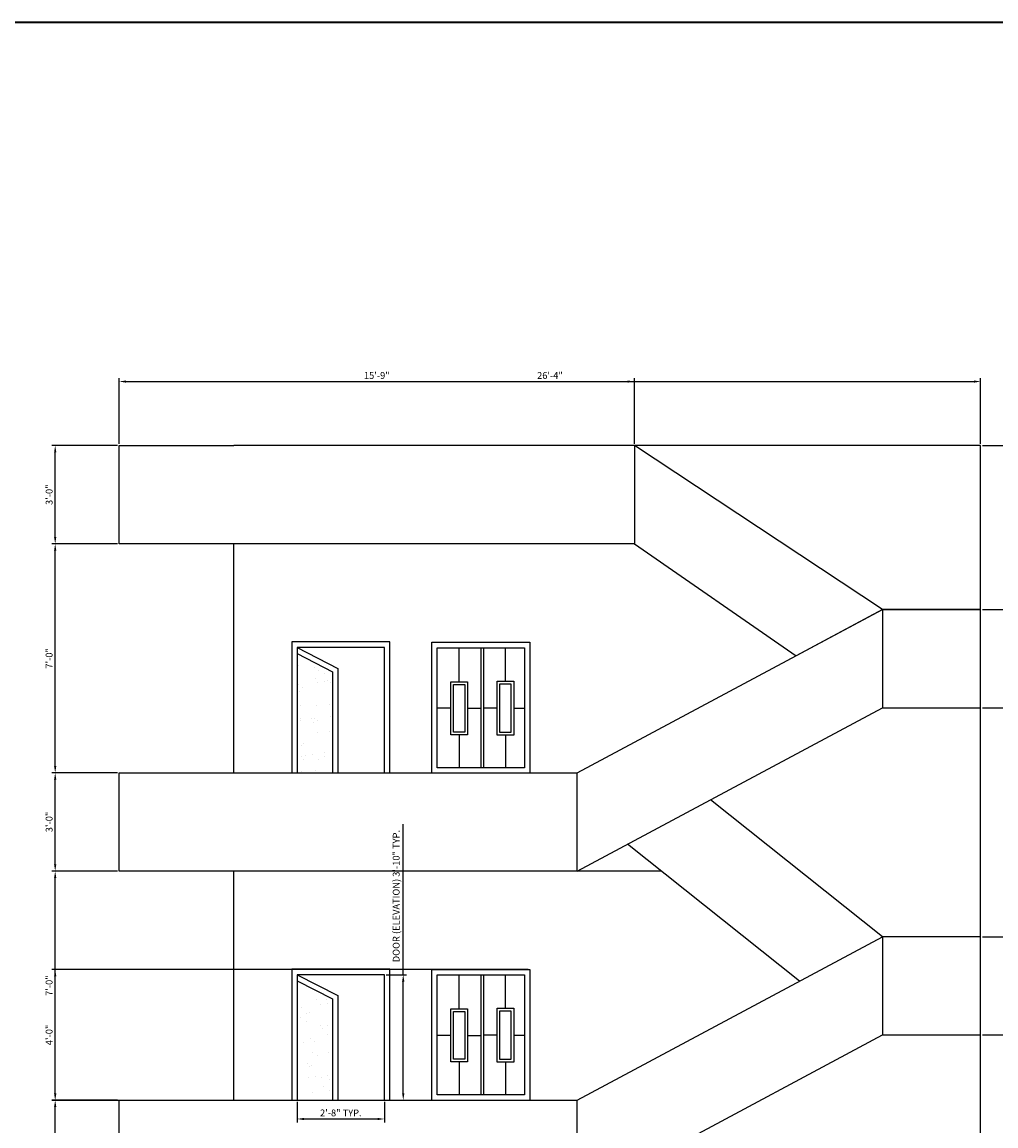
# Model space of a CAD drawing. Units: inches. Extents: x 2020 to 7901, y 1581 to 3943.
# Tile 7 of 17: x 2315 to 2672, y 2663 to 3067. Entities that reach past the tile are written whole.
import ezdxf

# ---------------------------------------------------------------- set-up
doc = ezdxf.new("R2010")
doc.units = ezdxf.units.IN
for name, color, linetype, lineweight in [('A-ANNO-DIMS', 2, 'Continuous', 18), ('A-ANNO-TTLB', 7, 'Continuous', 35), ('A-ELEV', 7, 'Continuous', 25), ('A-ELEV-PATT', 8, 'Continuous', 13)]:
    doc.layers.add(name, color=color, linetype=linetype, lineweight=lineweight)
doc.styles.get("Standard").update_dxf_attribs({"font": 'arial.ttf'})
doc.dimstyles.new('ISO-25', dxfattribs={"dimtxt": 2.5, "dimasz": 2.5, "dimexe": 1.25, "dimexo": 0.625, "dimtad": 1, "dimdec": 1, "dimlunit": 3, "dimtxsty": 'Standard', "dimcen": 2.5, "dimadec": 0, "dimazin": 0, "dimtfac": 1, "dimtdec": 1, "dimtmove": 0, "dimatfit": 3, "dimfxl": 1, "dimarcsym": 0})
pattern_1 = [(37.5, (-52.601, -26.04), (-0.320006, 9.788265), [0, -7.7216, 0, -8.636, 0, -8.255]), (7.5, (-52.601, -26.04), (8.990466, 14.3365), [0, -4.1656, 0, -6.9596, 0, -2.667]), (327.5, (-58.849, -26.04), (15.819847, 0.028744), [0, -2.54, 0, -9.144, 0, -11.938]), (317.5, (-58.85, -26.04), (15.27113, 4.458586), [0, -1.27, 0, -5.9944, 0, -6.858])]

# ---------------------------------------------------------------- blocks, each defined once
blk = doc.blocks.new('ELEV-DOOR')
for p, q in [((32, 46), (0, 46)), ((0, 46), (0, 0)), ((0, 46), (14.91, 38.33)), ((32, 0), (32, 46)), ((14.91, 38.33), (14.91, 0))]:
    blk.add_line(p, q)
blk = doc.blocks.new('*D29')
at = {"layer": 'A-ANNO-DIMS', "color": 0, "lineweight": -2, "transparency": 16777216}
for p, q in [((2454.54, 2717.95), (2454.54, 2773.1)), ((2448.26, 2717.95), (2455.79, 2717.95)), ((2454.54, 2674.45), (2454.54, 2715.45)), ((2448.26, 2671.95), (2455.79, 2671.95))]:
    blk.add_line(p, q, dxfattribs=at)
at = {"layer": 'A-ANNO-DIMS', "color": 0, "transparency": 16777216}
for points in [[(2454.12, 2715.45), (2454.96, 2715.45), (2454.54, 2717.95)], [(2454.12, 2674.45), (2454.96, 2674.45), (2454.54, 2671.95)]]:
    blk.add_solid(points, dxfattribs=at)
at = {"layer": 'DEFPOINTS', "color": 0, "transparency": 16777216}
for p in [(2447.64, 2717.95), (2454.54, 2717.95), (2447.64, 2671.95)]:
    blk.add_point(p, dxfattribs=at)
at = {"layer": 'A-ANNO-DIMS', "color": 0, "transparency": 16777216, "insert": (2452.27, 2746.77), "char_height": 2.5, "attachment_point": 5, "rotation": 90}
blk.add_mtext('DOOR (ELEVATION) 3\'-10" TYP.', dxfattribs=at)
blk = doc.blocks.new('*D30')
at = {"layer": 'A-ANNO-DIMS', "color": 0, "lineweight": -2, "transparency": 16777216}
for p, q in [((2415.64, 2671.32), (2415.64, 2663.8)), ((2447.64, 2671.32), (2447.64, 2663.8)), ((2418.14, 2665.05), (2445.14, 2665.05))]:
    blk.add_line(p, q, dxfattribs=at)
at = {"layer": 'A-ANNO-DIMS', "color": 0, "transparency": 16777216}
for points in [[(2418.14, 2665.46), (2418.14, 2664.63), (2415.64, 2665.05)], [(2445.14, 2665.46), (2445.14, 2664.63), (2447.64, 2665.05)]]:
    blk.add_solid(points, dxfattribs=at)
at = {"layer": 'DEFPOINTS', "color": 0, "transparency": 16777216}
for p in [(2415.64, 2671.95), (2447.64, 2671.95), (2447.64, 2665.05)]:
    blk.add_point(p, dxfattribs=at)
at = {"layer": 'A-ANNO-DIMS', "color": 0, "transparency": 16777216, "insert": (2431.64, 2666.95), "char_height": 2.5, "attachment_point": 5}
blk.add_mtext('2\'-8" TYP.', dxfattribs=at)
blk = doc.blocks.new('*D62')
at = {"layer": 'A-ANNO-DIMS', "color": 0, "lineweight": -2, "transparency": 16777216}
for p, q in [((2350.36, 2912.57), (2350.36, 2936.7)), ((2352.86, 2935.45), (2663.86, 2935.45)), ((2666.36, 2912.57), (2666.36, 2936.7))]:
    blk.add_line(p, q, dxfattribs=at)
at = {"layer": 'A-ANNO-DIMS', "color": 0, "transparency": 16777216}
for points in [[(2352.86, 2935.86), (2352.86, 2935.03), (2350.36, 2935.45)], [(2663.86, 2935.86), (2663.86, 2935.03), (2666.36, 2935.45)]]:
    blk.add_solid(points, dxfattribs=at)
at = {"layer": 'DEFPOINTS', "color": 0, "transparency": 16777216}
for p in [(2666.36, 2935.45), (2350.36, 2911.95), (2666.36, 2911.95)]:
    blk.add_point(p, dxfattribs=at)
at = {"layer": 'A-ANNO-DIMS', "color": 0, "transparency": 16777216, "insert": (2508.36, 2937.35), "char_height": 2.5, "attachment_point": 5}
blk.add_mtext('26\'-4"', dxfattribs=at)
blk = doc.blocks.new('*D63')
at = {"layer": 'A-ANNO-DIMS', "color": 0, "lineweight": -2, "transparency": 16777216}
for p, q in [((2666.99, 2911.95), (2728.83, 2911.95)), ((2727.58, 2490.45), (2727.58, 2909.45)), ((2666.99, 2487.95), (2728.83, 2487.95))]:
    blk.add_line(p, q, dxfattribs=at)
at = {"layer": 'A-ANNO-DIMS', "color": 0, "transparency": 16777216}
for points in [[(2727.17, 2909.45), (2728, 2909.45), (2727.58, 2911.95)], [(2727.17, 2490.45), (2728, 2490.45), (2727.58, 2487.95)]]:
    blk.add_solid(points, dxfattribs=at)
at = {"layer": 'DEFPOINTS', "color": 0, "transparency": 16777216}
for p in [(2666.36, 2911.95), (2727.58, 2911.95), (2666.36, 2487.95)]:
    blk.add_point(p, dxfattribs=at)
at = {"layer": 'A-ANNO-DIMS', "color": 0, "transparency": 16777216, "insert": (2725.68, 2699.95), "char_height": 2.5, "attachment_point": 5, "rotation": 90}
blk.add_mtext('35\'-4"', dxfattribs=at)
blk = doc.blocks.new('*D68')
at = {"layer": 'A-ANNO-DIMS', "color": 0, "lineweight": -2, "transparency": 16777216}
for p, q in [((2349.74, 2671.95), (2325.61, 2671.95)), ((2326.86, 2638.45), (2326.86, 2669.45)), ((2349.74, 2635.95), (2325.61, 2635.95))]:
    blk.add_line(p, q, dxfattribs=at)
at = {"layer": 'A-ANNO-DIMS', "color": 0, "transparency": 16777216}
for points in [[(2326.45, 2669.45), (2327.28, 2669.45), (2326.86, 2671.95)], [(2326.45, 2638.45), (2327.28, 2638.45), (2326.86, 2635.95)]]:
    blk.add_solid(points, dxfattribs=at)
at = {"layer": 'DEFPOINTS', "color": 0, "transparency": 16777216}
for p in [(2326.86, 2671.95), (2350.36, 2671.95), (2350.36, 2635.95)]:
    blk.add_point(p, dxfattribs=at)
at = {"layer": 'A-ANNO-DIMS', "color": 0, "transparency": 16777216, "insert": (2324.96, 2653.95), "char_height": 2.5, "attachment_point": 5, "rotation": 90}
blk.add_mtext('3\'-0"', dxfattribs=at)
blk = doc.blocks.new('*D69')
at = {"layer": 'A-ANNO-DIMS', "color": 0, "lineweight": -2, "transparency": 16777216}
for p, q in [((2349.74, 2755.95), (2325.61, 2755.95)), ((2326.86, 2674.45), (2326.86, 2753.45)), ((2349.74, 2671.95), (2325.61, 2671.95))]:
    blk.add_line(p, q, dxfattribs=at)
at = {"layer": 'A-ANNO-DIMS', "color": 0, "transparency": 16777216}
for points in [[(2326.45, 2753.45), (2327.28, 2753.45), (2326.86, 2755.95)], [(2326.45, 2674.45), (2327.28, 2674.45), (2326.86, 2671.95)]]:
    blk.add_solid(points, dxfattribs=at)
at = {"layer": 'DEFPOINTS', "color": 0, "transparency": 16777216}
for p in [(2326.86, 2755.95), (2350.36, 2755.95), (2350.36, 2671.95)]:
    blk.add_point(p, dxfattribs=at)
at = {"layer": 'A-ANNO-DIMS', "color": 0, "transparency": 16777216, "insert": (2324.96, 2713.95), "char_height": 2.5, "attachment_point": 5, "rotation": 90}
blk.add_mtext('7\'-0"', dxfattribs=at)
blk = doc.blocks.new('*D70')
at = {"layer": 'A-ANNO-DIMS', "color": 0, "lineweight": -2, "transparency": 16777216}
for p, q in [((2349.74, 2791.95), (2325.61, 2791.95)), ((2326.86, 2758.45), (2326.86, 2789.45)), ((2349.74, 2755.95), (2325.61, 2755.95))]:
    blk.add_line(p, q, dxfattribs=at)
at = {"layer": 'A-ANNO-DIMS', "color": 0, "transparency": 16777216}
for points in [[(2326.45, 2789.45), (2327.28, 2789.45), (2326.86, 2791.95)], [(2326.45, 2758.45), (2327.28, 2758.45), (2326.86, 2755.95)]]:
    blk.add_solid(points, dxfattribs=at)
at = {"layer": 'DEFPOINTS', "color": 0, "transparency": 16777216}
for p in [(2326.86, 2791.95), (2350.36, 2791.95), (2350.36, 2755.95)]:
    blk.add_point(p, dxfattribs=at)
at = {"layer": 'A-ANNO-DIMS', "color": 0, "transparency": 16777216, "insert": (2324.96, 2773.95), "char_height": 2.5, "attachment_point": 5, "rotation": 90}
blk.add_mtext('3\'-0"', dxfattribs=at)
blk = doc.blocks.new('*D71')
at = {"layer": 'A-ANNO-DIMS', "color": 0, "lineweight": -2, "transparency": 16777216}
for p, q in [((2349.74, 2875.95), (2325.61, 2875.95)), ((2326.86, 2794.45), (2326.86, 2873.45)), ((2349.74, 2791.95), (2325.61, 2791.95))]:
    blk.add_line(p, q, dxfattribs=at)
at = {"layer": 'A-ANNO-DIMS', "color": 0, "transparency": 16777216}
for points in [[(2326.45, 2873.45), (2327.28, 2873.45), (2326.86, 2875.95)], [(2326.45, 2794.45), (2327.28, 2794.45), (2326.86, 2791.95)]]:
    blk.add_solid(points, dxfattribs=at)
at = {"layer": 'DEFPOINTS', "color": 0, "transparency": 16777216}
for p in [(2326.86, 2875.95), (2350.36, 2875.95), (2350.36, 2791.95)]:
    blk.add_point(p, dxfattribs=at)
at = {"layer": 'A-ANNO-DIMS', "color": 0, "transparency": 16777216, "insert": (2324.96, 2833.95), "char_height": 2.5, "attachment_point": 5, "rotation": 90}
blk.add_mtext('7\'-0"', dxfattribs=at)
blk = doc.blocks.new('*D72')
at = {"layer": 'A-ANNO-DIMS', "color": 0, "lineweight": -2, "transparency": 16777216}
for p, q in [((2349.74, 2911.95), (2325.61, 2911.95)), ((2326.86, 2878.45), (2326.86, 2909.45)), ((2349.74, 2875.95), (2325.61, 2875.95))]:
    blk.add_line(p, q, dxfattribs=at)
at = {"layer": 'A-ANNO-DIMS', "color": 0, "transparency": 16777216}
for points in [[(2326.45, 2909.45), (2327.28, 2909.45), (2326.86, 2911.95)], [(2326.45, 2878.45), (2327.28, 2878.45), (2326.86, 2875.95)]]:
    blk.add_solid(points, dxfattribs=at)
at = {"layer": 'DEFPOINTS', "color": 0, "transparency": 16777216}
for p in [(2326.86, 2911.95), (2350.36, 2911.95), (2350.36, 2875.95)]:
    blk.add_point(p, dxfattribs=at)
at = {"layer": 'A-ANNO-DIMS', "color": 0, "transparency": 16777216, "insert": (2324.96, 2893.95), "char_height": 2.5, "attachment_point": 5, "rotation": 90}
blk.add_mtext('3\'-0"', dxfattribs=at)
blk = doc.blocks.new('*D150')
at = {"layer": 'A-ANNO-DIMS', "color": 0, "lineweight": -2, "transparency": 16777216}
for p, q in [((2666.99, 2695.85), (2728.83, 2695.85)), ((2727.58, 2614.35), (2727.58, 2693.35)), ((2666.99, 2611.85), (2728.83, 2611.85))]:
    blk.add_line(p, q, dxfattribs=at)
at = {"layer": 'A-ANNO-DIMS', "color": 0, "transparency": 16777216}
for points in [[(2727.17, 2693.35), (2728, 2693.35), (2727.58, 2695.85)], [(2727.17, 2614.35), (2728, 2614.35), (2727.58, 2611.85)]]:
    blk.add_solid(points, dxfattribs=at)
at = {"layer": 'DEFPOINTS', "color": 0, "transparency": 16777216}
for p in [(2666.36, 2695.85), (2727.58, 2695.85), (2666.36, 2611.85)]:
    blk.add_point(p, dxfattribs=at)
at = {"layer": 'A-ANNO-DIMS', "color": 0, "transparency": 16777216, "insert": (2725.68, 2653.85), "char_height": 2.5, "attachment_point": 5, "rotation": 90}
blk.add_mtext('7\'-0"', dxfattribs=at)
blk = doc.blocks.new('*D151')
at = {"layer": 'A-ANNO-DIMS', "color": 0, "lineweight": -2, "transparency": 16777216}
for p, q in [((2666.99, 2731.85), (2728.83, 2731.85)), ((2727.58, 2698.35), (2727.58, 2729.35)), ((2666.99, 2695.85), (2728.83, 2695.85))]:
    blk.add_line(p, q, dxfattribs=at)
at = {"layer": 'A-ANNO-DIMS', "color": 0, "transparency": 16777216}
for points in [[(2727.17, 2729.35), (2728, 2729.35), (2727.58, 2731.85)], [(2727.17, 2698.35), (2728, 2698.35), (2727.58, 2695.85)]]:
    blk.add_solid(points, dxfattribs=at)
at = {"layer": 'DEFPOINTS', "color": 0, "transparency": 16777216}
for p in [(2666.36, 2731.85), (2727.58, 2731.85), (2666.36, 2695.85)]:
    blk.add_point(p, dxfattribs=at)
at = {"layer": 'A-ANNO-DIMS', "color": 0, "transparency": 16777216, "insert": (2725.68, 2713.85), "char_height": 2.5, "attachment_point": 5, "rotation": 90}
blk.add_mtext('3\'-0"', dxfattribs=at)
blk = doc.blocks.new('*D152')
at = {"layer": 'A-ANNO-DIMS', "color": 0, "lineweight": -2, "transparency": 16777216}
for p, q in [((2666.99, 2815.83), (2728.83, 2815.83)), ((2727.58, 2734.35), (2727.58, 2813.33)), ((2666.99, 2731.85), (2728.83, 2731.85))]:
    blk.add_line(p, q, dxfattribs=at)
at = {"layer": 'A-ANNO-DIMS', "color": 0, "transparency": 16777216}
for points in [[(2727.17, 2813.33), (2728, 2813.33), (2727.58, 2815.83)], [(2727.17, 2734.35), (2728, 2734.35), (2727.58, 2731.85)]]:
    blk.add_solid(points, dxfattribs=at)
at = {"layer": 'DEFPOINTS', "color": 0, "transparency": 16777216}
for p in [(2666.36, 2815.83), (2727.58, 2815.83), (2666.36, 2731.85)]:
    blk.add_point(p, dxfattribs=at)
at = {"layer": 'A-ANNO-DIMS', "color": 0, "transparency": 16777216, "insert": (2725.68, 2773.84), "char_height": 2.5, "attachment_point": 5, "rotation": 90}
blk.add_mtext('7\'-0"', dxfattribs=at)
blk = doc.blocks.new('*D153')
at = {"layer": 'A-ANNO-DIMS', "color": 0, "lineweight": -2, "transparency": 16777216}
for p, q in [((2666.99, 2851.83), (2728.83, 2851.83)), ((2727.58, 2818.33), (2727.58, 2849.33)), ((2666.99, 2815.83), (2728.83, 2815.83))]:
    blk.add_line(p, q, dxfattribs=at)
at = {"layer": 'A-ANNO-DIMS', "color": 0, "transparency": 16777216}
for points in [[(2727.17, 2849.33), (2728, 2849.33), (2727.58, 2851.83)], [(2727.17, 2818.33), (2728, 2818.33), (2727.58, 2815.83)]]:
    blk.add_solid(points, dxfattribs=at)
at = {"layer": 'DEFPOINTS', "color": 0, "transparency": 16777216}
for p in [(2666.36, 2851.83), (2727.58, 2851.83), (2666.36, 2815.83)]:
    blk.add_point(p, dxfattribs=at)
at = {"layer": 'A-ANNO-DIMS', "color": 0, "transparency": 16777216, "insert": (2725.68, 2833.83), "char_height": 2.5, "attachment_point": 5, "rotation": 90}
blk.add_mtext('3\'-0"', dxfattribs=at)
blk = doc.blocks.new('*D154')
at = {"layer": 'A-ANNO-DIMS', "color": 0, "lineweight": -2, "transparency": 16777216}
for p, q in [((2666.99, 2911.95), (2728.83, 2911.95)), ((2727.58, 2854.33), (2727.58, 2909.45)), ((2666.99, 2851.83), (2728.83, 2851.83))]:
    blk.add_line(p, q, dxfattribs=at)
at = {"layer": 'A-ANNO-DIMS', "color": 0, "transparency": 16777216}
for points in [[(2727.17, 2909.45), (2728, 2909.45), (2727.58, 2911.95)], [(2727.17, 2854.33), (2728, 2854.33), (2727.58, 2851.83)]]:
    blk.add_solid(points, dxfattribs=at)
at = {"layer": 'DEFPOINTS', "color": 0, "transparency": 16777216}
for p in [(2666.36, 2911.95), (2727.58, 2911.95), (2666.36, 2851.83)]:
    blk.add_point(p, dxfattribs=at)
at = {"layer": 'A-ANNO-DIMS', "color": 0, "transparency": 16777216, "insert": (2725.68, 2881.89), "char_height": 2.5, "attachment_point": 5, "rotation": 90}
blk.add_mtext('5\'-0"', dxfattribs=at)
blk = doc.blocks.new('*D155')
at = {"layer": 'A-ANNO-DIMS', "color": 0, "lineweight": -2, "transparency": 16777216}
for p, q in [((2350.36, 2912.57), (2350.36, 2936.7)), ((2352.86, 2935.45), (2536.82, 2935.45)), ((2539.32, 2912.57), (2539.32, 2936.7))]:
    blk.add_line(p, q, dxfattribs=at)
at = {"layer": 'A-ANNO-DIMS', "color": 0, "transparency": 16777216}
for points in [[(2352.86, 2935.86), (2352.86, 2935.03), (2350.36, 2935.45)], [(2536.82, 2935.86), (2536.82, 2935.03), (2539.32, 2935.45)]]:
    blk.add_solid(points, dxfattribs=at)
at = {"layer": 'DEFPOINTS', "color": 0, "transparency": 16777216}
for p in [(2539.32, 2935.45), (2350.36, 2911.95), (2539.32, 2911.95)]:
    blk.add_point(p, dxfattribs=at)
at = {"layer": 'A-ANNO-DIMS', "color": 0, "transparency": 16777216, "insert": (2444.84, 2937.35), "char_height": 2.5, "attachment_point": 5}
blk.add_mtext('15\'-9"', dxfattribs=at)
blk = doc.blocks.new('*D158')
at = {"layer": 'A-ANNO-DIMS', "color": 0, "lineweight": -2, "transparency": 16777216}
for p, q in [((2500.37, 2719.87), (2325.61, 2719.87)), ((2326.86, 2674.37), (2326.86, 2717.37)), ((2500.37, 2671.87), (2325.61, 2671.87))]:
    blk.add_line(p, q, dxfattribs=at)
at = {"layer": 'A-ANNO-DIMS', "color": 0, "transparency": 16777216}
for points in [[(2326.45, 2717.37), (2327.28, 2717.37), (2326.86, 2719.87)], [(2326.45, 2674.37), (2327.28, 2674.37), (2326.86, 2671.87)]]:
    blk.add_solid(points, dxfattribs=at)
at = {"layer": 'DEFPOINTS', "color": 0, "transparency": 16777216}
for p in [(2326.86, 2719.87), (2500.99, 2719.87), (2500.99, 2671.87)]:
    blk.add_point(p, dxfattribs=at)
at = {"layer": 'A-ANNO-DIMS', "color": 0, "transparency": 16777216, "insert": (2324.96, 2695.87), "char_height": 2.5, "attachment_point": 5, "rotation": 90}
blk.add_mtext('4\'-0"', dxfattribs=at)

msp = doc.modelspace()

# ---------------------------------------------------------------- hatches: boundary and pattern name
at = {"layer": 'A-ELEV-PATT'}
h = msp.add_hatch(dxfattribs=at)
h.set_pattern_fill('AR-SAND', color=256, scale=0.2)
h.set_pattern_definition(pattern_1)
h.paths.add_polyline_path([(2428.55, 2829.06), (2415.64, 2835.7), (2415.64, 2791.95), (2428.55, 2791.95)])
h = msp.add_hatch(dxfattribs=at)
h.set_pattern_fill('AR-SAND', color=256, scale=0.2)
h.set_pattern_definition(pattern_1)
h.paths.add_polyline_path([(2428.55, 2709.06), (2415.64, 2715.7), (2415.64, 2671.95), (2428.55, 2671.95)])

# ---------------------------------------------------------------- linework, layer by layer
at = {"layer": 'A-ANNO-TTLB'}
msp.add_lwpolyline([(2019.8, 3067.25), (4199.03, 3067.25), (4199.03, 1580.73), (2019.8, 1580.73)], close=True, dxfattribs=at)
at = {"layer": 'A-ELEV'}
for p, q in [((2350.36, 2875.95), (2350.36, 2911.95)), ((2350.36, 2911.95), (2392.36, 2911.95)), ((2666.36, 2911.95), (2392.36, 2911.95)), ((2539.32, 2911.95), (2539.32, 2875.95)), ((2630.36, 2851.83), (2539.32, 2911.95)), ((2666.36, 2487.95), (2666.36, 2911.95)), ((2392.36, 2875.95), (2350.36, 2875.95)), ((2392.36, 2791.95), (2392.36, 2875.95)), ((2539.32, 2875.95), (2392.36, 2875.95)), ((2539.32, 2875.95), (2598.62, 2834.86)), ((2518.36, 2791.95), (2630.36, 2851.83)), ((2630.36, 2851.83), (2598.62, 2834.86)), ((2630.36, 2851.83), (2598.62, 2834.86)), ((2666.36, 2851.83), (2630.36, 2851.83)), ((2630.36, 2851.83), (2630.36, 2815.83)), ((2630.36, 2851.83), (2666.36, 2851.83)), ((2475.07, 2825.39), (2475.07, 2837.83)), ((2482.99, 2837.83), (2482.99, 2793.83)), ((2483.99, 2837.83), (2483.99, 2793.83)), ((2492.02, 2825.62), (2492.02, 2837.83)), ((2415.64, 2835.7), (2428.55, 2829.06)), ((2428.55, 2829.06), (2428.55, 2791.95)), ((2471.99, 2815.65), (2466.99, 2815.65)), ((2478.15, 2815.65), (2482.99, 2815.65)), ((2488.99, 2815.71), (2483.99, 2815.71)), ((2495.06, 2815.71), (2498.99, 2815.71)), ((2518.36, 2755.95), (2630.36, 2815.83)), ((2630.36, 2815.83), (2666.36, 2815.83)), ((2475.07, 2805.91), (2475.07, 2793.83)), ((2492.02, 2805.79), (2492.02, 2793.83)), ((2350.36, 2755.95), (2350.36, 2791.95)), ((2350.36, 2791.95), (2518.36, 2791.95)), ((2518.36, 2755.95), (2518.36, 2791.95)), ((2630.36, 2731.85), (2567.22, 2782.07)), ((2599.91, 2715.56), (2536.77, 2765.79)), ((2392.36, 2755.95), (2350.36, 2755.95)), ((2392.36, 2671.95), (2392.36, 2755.95)), ((2549.14, 2755.95), (2392.36, 2755.95)), ((2518.36, 2671.95), (2630.36, 2731.85)), ((2666.36, 2731.85), (2630.36, 2731.85)), ((2630.36, 2731.85), (2630.36, 2695.85)), ((2475.07, 2705.43), (2475.07, 2717.87)), ((2482.99, 2717.87), (2482.99, 2673.87)), ((2483.99, 2717.87), (2483.99, 2673.87)), ((2492.02, 2705.66), (2492.02, 2717.87)), ((2415.64, 2715.7), (2428.55, 2709.06)), ((2428.55, 2709.06), (2428.55, 2671.95)), ((2471.99, 2695.69), (2466.99, 2695.69)), ((2478.15, 2695.69), (2482.99, 2695.69)), ((2488.99, 2695.75), (2483.99, 2695.75)), ((2495.06, 2695.75), (2498.99, 2695.75)), ((2518.36, 2635.95), (2630.36, 2695.85)), ((2630.36, 2695.85), (2666.36, 2695.85)), ((2475.07, 2685.95), (2475.07, 2673.87)), ((2492.02, 2685.83), (2492.02, 2673.87)), ((2350.36, 2635.95), (2350.36, 2671.95)), ((2350.36, 2671.95), (2518.36, 2671.95)), ((2518.36, 2505.95), (2518.36, 2671.95))]:
    msp.add_line(p, q, dxfattribs=at)
for points in [[(2449.64, 2791.95), (2449.64, 2839.95), (2413.64, 2839.95), (2413.64, 2791.95)], [(2449.64, 2671.95), (2449.64, 2719.95), (2413.64, 2719.95), (2413.64, 2671.95)]]:
    msp.add_lwpolyline(points, dxfattribs=at)
for points in [[(2464.99, 2839.83), (2500.99, 2839.83), (2500.99, 2791.83), (2464.99, 2791.83)], [(2466.99, 2837.83), (2498.99, 2837.83), (2498.99, 2793.83), (2466.99, 2793.83)], [(2471.99, 2825.39), (2478.15, 2825.39), (2478.15, 2805.91), (2471.99, 2805.91)], [(2488.99, 2825.62), (2495.06, 2825.62), (2495.06, 2805.79), (2488.99, 2805.79)], [(2472.99, 2824.39), (2477.15, 2824.39), (2477.15, 2806.91), (2472.99, 2806.91)], [(2489.99, 2824.62), (2494.06, 2824.62), (2494.06, 2806.79), (2489.99, 2806.79)], [(2464.99, 2719.87), (2500.99, 2719.87), (2500.99, 2671.87), (2464.99, 2671.87)], [(2466.99, 2717.87), (2498.99, 2717.87), (2498.99, 2673.87), (2466.99, 2673.87)], [(2471.99, 2705.43), (2478.15, 2705.43), (2478.15, 2685.95), (2471.99, 2685.95)], [(2472.99, 2704.43), (2477.15, 2704.43), (2477.15, 2686.95), (2472.99, 2686.95)], [(2488.99, 2705.66), (2495.06, 2705.66), (2495.06, 2685.83), (2488.99, 2685.83)], [(2489.99, 2704.66), (2494.06, 2704.66), (2494.06, 2686.83), (2489.99, 2686.83)]]:
    msp.add_lwpolyline(points, close=True, dxfattribs=at)

# ---------------------------------------------------------------- block references
for p in [(2415.64, 2791.95), (2415.64, 2671.95)]:
    msp.add_blockref('ELEV-DOOR', p, dxfattribs=at)

# ---------------------------------------------------------------- dimensions: what is measured, and where the dimension line sits
at = {"layer": 'A-ANNO-DIMS'}
for base, p2, picture, middle in [((2666.36, 2935.45), (2666.36, 2911.95), '*D62', (2508.36, 2937.35)), ((2539.32, 2935.45), (2539.32, 2911.95), '*D155', (2444.84, 2937.35))]:
    dim = msp.add_linear_dim(base=base, p1=(2350.36, 2911.95), p2=p2, dimstyle='ISO-25', override={"dimdec": 1, "dimlfac": 1, "dimrnd": 0, "dimzin": 1, "dimdsep": 46, "dimlunit": 4, "dimfrac": 2}, dxfattribs=at)
    dim.commit()
    dim.dimension.update_dxf_attribs({"geometry": picture, "text_midpoint": middle})
for base, p1, p2, picture, middle in [((2326.86, 2911.95), (2350.36, 2875.95), (2350.36, 2911.95), '*D72', (2324.96, 2893.95)), ((2727.58, 2911.95), (2666.36, 2487.95), (2666.36, 2911.95), '*D63', (2725.68, 2699.95)), ((2727.58, 2911.95), (2666.36, 2851.83), (2666.36, 2911.95), '*D154', (2725.68, 2881.89)), ((2326.86, 2875.95), (2350.36, 2791.95), (2350.36, 2875.95), '*D71', (2324.96, 2833.95)), ((2727.58, 2851.83), (2666.36, 2815.83), (2666.36, 2851.83), '*D153', (2725.68, 2833.83)), ((2727.58, 2815.83), (2666.36, 2731.85), (2666.36, 2815.83), '*D152', (2725.68, 2773.84)), ((2326.86, 2791.95), (2350.36, 2755.95), (2350.36, 2791.95), '*D70', (2324.96, 2773.95)), ((2326.86, 2755.95), (2350.36, 2671.95), (2350.36, 2755.95), '*D69', (2324.96, 2713.95)), ((2727.58, 2731.85), (2666.36, 2695.85), (2666.36, 2731.85), '*D151', (2725.68, 2713.85)), ((2326.86, 2719.87), (2500.99, 2671.87), (2500.99, 2719.87), '*D158', (2324.96, 2695.87)), ((2727.58, 2695.85), (2666.36, 2611.85), (2666.36, 2695.85), '*D150', (2725.68, 2653.85)), ((2326.86, 2671.95), (2350.36, 2635.95), (2350.36, 2671.95), '*D68', (2324.96, 2653.95))]:
    dim = msp.add_linear_dim(base=base, p1=p1, p2=p2, angle=90, dimstyle='ISO-25', override={"dimdec": 1, "dimlfac": 1, "dimrnd": 0, "dimzin": 1, "dimdsep": 46, "dimlunit": 4, "dimfrac": 2}, dxfattribs=at)
    dim.commit()
    dim.dimension.update_dxf_attribs({"geometry": picture, "text_midpoint": middle})
dim = msp.add_linear_dim(base=(2454.54, 2717.95), p1=(2447.64, 2671.95), p2=(2447.64, 2717.95), angle=90, text='DOOR (ELEVATION) <> TYP.', dimstyle='ISO-25', override={"dimdec": 1, "dimrnd": 0, "dimzin": 1, "dimlunit": 4, "dimfrac": 2}, dxfattribs=at)
dim.commit()
dim.dimension.update_dxf_attribs({"geometry": '*D29', "text_midpoint": (2452.27, 2746.77)})
dim = msp.add_linear_dim(base=(2447.64, 2665.05), p1=(2415.64, 2671.95), p2=(2447.64, 2671.95), text='<> TYP.', dimstyle='ISO-25', override={"dimdec": 1, "dimrnd": 0, "dimzin": 1, "dimlunit": 4, "dimfrac": 2}, dxfattribs=at)
dim.commit()
dim.dimension.update_dxf_attribs({"geometry": '*D30', "text_midpoint": (2431.64, 2666.95)})

doc.saveas('drawing.dxf')
